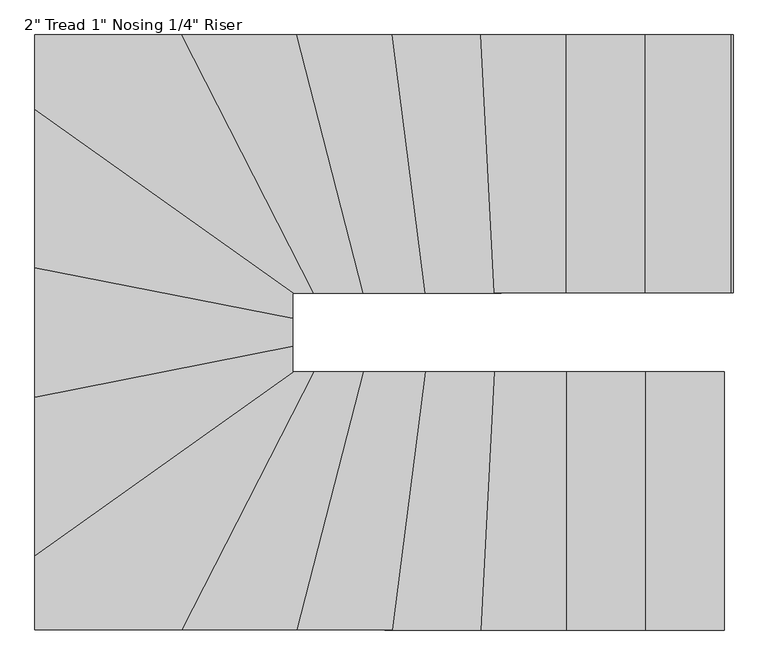
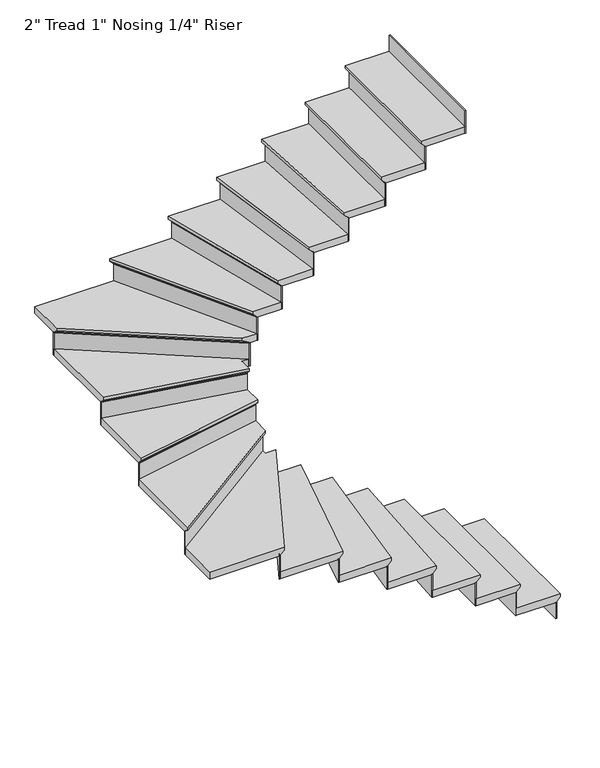
"""IFC4 building model written with IfcOpenShell, lengths in millimetres: stair flight geometry."""

from ifc_helpers import new_model, si_unit, origin, place, context, project, spatial, faceted_brep, source, transform, mapped, element, save


def stair_flight_e7c1aa98(model_context):
    return source(origin(), model_context, "Body", "Brep", [
        faceted_brep([(-14092.4170266, 7781.0465295, 150.2833333), (-14092.4170266, 7781.0465295, 169.3333333), (-14092.4170266, 6866.6465295, 169.3333333), (-14092.4170266, 6866.6465295, 150.2833333), (-14117.8170266, 7781.0465295, 124.8833333), (-14117.8170266, 6866.6465295, 124.8833333), (-14397.2170266, 7781.0465295, 169.3333333), (-14397.2170266, 6866.6465295, 169.3333333), (-14117.8170266, 6866.6465295, 118.5333333), (-14397.2170266, 6866.6465295, 118.5333333), (-14397.2170266, 7781.0465295, 118.5333333), (-14117.8170266, 7781.0465295, 118.5333333)], [[[0, 1, 2, 3]], [[4, 0, 3, 5]], [[2, 1, 6, 7]], [[8, 9, 10, 11]], [[2, 7, 9, 8, 5, 3]], [[8, 11, 4, 5]], [[6, 1, 0, 4, 11, 10]], [[7, 6, 10, 9]]]),
        faceted_brep([(-14117.8170266, 7781.0465295, 118.5333333), (-14117.8170266, 7781.0465295, 0.0), (-14124.1670266, 7781.0465295, 0.0), (-14124.1670266, 7781.0465295, 118.5333333), (-14117.8170266, 6866.6465295, 118.5333333), (-14124.1670266, 6866.6465295, 118.5333333), (-14124.1670266, 6866.6465295, 0.0), (-14117.8170266, 6866.6465295, 0.0)], [[[0, 1, 2, 3]], [[4, 5, 6, 7]], [[1, 0, 4, 7]], [[2, 1, 7, 6]], [[3, 2, 6, 5]], [[0, 3, 5, 4]]]),
        faceted_brep([(-14397.2170266, 7781.0465295, 287.8666667), (-14397.2170266, 7781.0465295, 118.5333333), (-14403.5670266, 7781.0465295, 118.5333333), (-14403.5670266, 7781.0465295, 287.8666667), (-14397.2170266, 6866.6465295, 287.8666667), (-14403.5670266, 6866.6465295, 287.8666667), (-14403.5670266, 6866.6465295, 118.5333333), (-14397.2170266, 6866.6465295, 118.5333333)], [[[0, 1, 2, 3]], [[4, 5, 6, 7]], [[1, 0, 4, 7]], [[2, 1, 7, 6]], [[3, 2, 6, 5]], [[0, 3, 5, 4]]]),
        faceted_brep([(-14371.8170266, 6866.6465295, 338.6666667), (-14371.8170266, 7781.0465295, 338.6666667), (-14676.6170266, 7781.0465295, 338.6666667), (-14676.6170266, 6866.6465295, 338.6666667), (-14397.2170266, 6866.6465295, 287.8666667), (-14676.6170266, 6866.6465295, 287.8666667), (-14676.6170266, 7781.0465295, 287.8666667), (-14397.2170266, 7781.0465295, 287.8666667), (-14397.2170266, 6866.6465295, 294.2166667), (-14371.8170266, 6866.6465295, 319.6166667), (-14397.2170266, 7781.0465295, 294.2166667), (-14371.8170266, 7781.0465295, 319.6166667)], [[[0, 1, 2, 3]], [[4, 5, 6, 7]], [[0, 3, 5, 4, 8, 9]], [[4, 7, 10, 8]], [[2, 1, 11, 10, 7, 6]], [[3, 2, 6, 5]], [[11, 1, 0, 9]], [[10, 11, 9, 8]]]),
        faceted_brep([(-14676.6170266, 7781.0465295, 457.2), (-14676.6170266, 7781.0465295, 287.8666667), (-14682.9670266, 7781.0465295, 287.8666667), (-14682.9670266, 7781.0465295, 457.2), (-14676.6170266, 6866.6465295, 457.2), (-14682.9670266, 6866.6465295, 457.2), (-14682.9670266, 6866.6465295, 287.8666667), (-14676.6170266, 6866.6465295, 287.8666667)], [[[0, 1, 2, 3]], [[4, 5, 6, 7]], [[1, 0, 4, 7]], [[2, 1, 7, 6]], [[3, 2, 6, 5]], [[0, 3, 5, 4]]]),
        faceted_brep([(-14651.2170266, 6866.6465295, 508.0), (-14651.2170266, 7781.0465295, 508.0), (-14932.284188, 7781.0465295, 508.0), (-14979.8184584, 6866.6465295, 508.0), (-14676.6170266, 6866.6465295, 457.2), (-14979.8184584, 6866.6465295, 457.2), (-14932.284188, 7781.0465295, 457.2), (-14676.6170266, 7781.0465295, 457.2), (-14676.6170266, 6866.6465295, 463.55), (-14651.2170266, 6866.6465295, 488.95), (-14676.6170266, 7781.0465295, 463.55), (-14651.2170266, 7781.0465295, 488.95)], [[[0, 1, 2, 3]], [[4, 5, 6, 7]], [[0, 3, 5, 4, 8, 9]], [[4, 7, 10, 8]], [[2, 1, 11, 10, 7, 6]], [[3, 2, 6, 5]], [[11, 1, 0, 9]], [[10, 11, 9, 8]]]),
        faceted_brep([(-14932.284188, 7781.0465295, 626.5333333), (-14932.284188, 7781.0465295, 457.2), (-14938.6427622, 7781.0465295, 457.2), (-14938.6427622, 7781.0465295, 626.5333333), (-14979.8184584, 6866.6465295, 626.5333333), (-14986.1770326, 6866.6465295, 626.5333333), (-14986.1770326, 6866.6465295, 457.2), (-14979.8184584, 6866.6465295, 457.2)], [[[0, 1, 2, 3]], [[4, 5, 6, 7]], [[1, 0, 4, 7]], [[2, 1, 7, 6]], [[3, 2, 6, 5]], [[0, 3, 5, 4]]]),
        faceted_brep([(-14954.3841618, 6866.6465295, 677.3333333), (-14906.8498914, 7781.0465295, 677.3333333), (-15176.4508879, 7781.0465295, 677.3333333), (-15294.8069395, 6866.6465295, 677.3333333), (-14979.8184584, 6866.6465295, 626.5333333), (-15294.8069395, 6866.6465295, 626.5333333), (-15176.4508879, 7781.0465295, 626.5333333), (-14932.284188, 7781.0465295, 626.5333333), (-14979.8184584, 6866.6465295, 632.8833333), (-14954.3841618, 6866.6465295, 658.2833333), (-14932.284188, 7781.0465295, 632.8833333), (-14906.8498914, 7781.0465295, 658.2833333)], [[[0, 1, 2, 3]], [[4, 5, 6, 7]], [[0, 3, 5, 4, 8, 9]], [[4, 7, 10, 8]], [[2, 1, 11, 10, 7, 6]], [[3, 2, 6, 5]], [[11, 1, 0, 9]], [[10, 11, 9, 8]]]),
        faceted_brep([(-15176.4508879, 7781.0465295, 795.8666667), (-15176.4508879, 7781.0465295, 626.5333333), (-15182.8538596, 7781.0465295, 626.5333333), (-15182.8538596, 7781.0465295, 795.8666667), (-15294.8069395, 6866.6465295, 795.8666667), (-15301.2099113, 6866.6465295, 795.8666667), (-15301.2099113, 6866.6465295, 626.5333333), (-15294.8069395, 6866.6465295, 626.5333333)], [[[0, 1, 2, 3]], [[4, 5, 6, 7]], [[1, 0, 4, 7]], [[2, 1, 7, 6]], [[3, 2, 6, 5]], [[0, 3, 5, 4]]]),
        faceted_brep([(-15269.1950524, 6866.6465295, 846.6666667), (-15150.8390007, 7781.0465295, 846.6666667), (-15398.0781103, 7781.0465295, 846.6666667), (-15633.2085577, 6866.6465295, 846.6666667), (-15294.8069395, 6866.6465295, 795.8666667), (-15633.2085577, 6866.6465295, 795.8666667), (-15398.0781103, 7781.0465295, 795.8666667), (-15176.4508879, 7781.0465295, 795.8666667), (-15294.8069395, 6866.6465295, 802.2166667), (-15269.1950524, 6866.6465295, 827.6166667), (-15176.4508879, 7781.0465295, 802.2166667), (-15150.8390007, 7781.0465295, 827.6166667)], [[[0, 1, 2, 3]], [[4, 5, 6, 7]], [[0, 3, 5, 4, 8, 9]], [[4, 7, 10, 8]], [[2, 1, 11, 10, 7, 6]], [[3, 2, 6, 5]], [[11, 1, 0, 9]], [[10, 11, 9, 8]]]),
        faceted_brep([(-15398.0781103, 7781.0465295, 965.2), (-15398.0781103, 7781.0465295, 795.8666667), (-15404.6346872, 7781.0465295, 795.8666667), (-15404.6346872, 7781.0465295, 965.2), (-15633.2085577, 6866.6465295, 965.2), (-15639.7651346, 6866.6465295, 965.2), (-15639.7651346, 6866.6465295, 795.8666667), (-15633.2085577, 6866.6465295, 795.8666667)], [[[0, 1, 2, 3]], [[4, 5, 6, 7]], [[1, 0, 4, 7]], [[2, 1, 7, 6]], [[3, 2, 6, 5]], [[0, 3, 5, 4]]]),
        faceted_brep([(-15606.9822503, 6866.6465295, 1016.0), (-15371.8518029, 7781.0465295, 1016.0), (-15574.4247464, 7781.0465295, 1016.0), (-16043.2493677, 6866.6465295, 1016.0), (-15633.2085577, 6866.6465295, 965.2), (-16043.2493677, 6866.6465295, 965.2), (-15574.4247464, 7781.0465295, 965.2), (-15398.0781103, 7781.0465295, 965.2), (-15633.2085577, 6866.6465295, 971.55), (-15606.9822503, 6866.6465295, 996.95), (-15398.0781103, 7781.0465295, 971.55), (-15371.8518029, 7781.0465295, 996.95)], [[[0, 1, 2, 3]], [[4, 5, 6, 7]], [[0, 3, 5, 4, 8, 9]], [[4, 7, 10, 8]], [[2, 1, 11, 10, 7, 6]], [[3, 2, 6, 5]], [[11, 1, 0, 9]], [[10, 11, 9, 8]]]),
        faceted_brep([(-15574.4247464, 7781.0465295, 1134.5333333), (-15574.4247464, 7781.0465295, 965.2), (-15581.5607295, 7781.0465295, 965.2), (-15581.5607295, 7781.0465295, 1134.5333333), (-16043.2493677, 6866.6465295, 1134.5333333), (-16050.3853509, 6866.6465295, 1134.5333333), (-16050.3853509, 6866.6465295, 965.2), (-16043.2493677, 6866.6465295, 965.2)], [[[0, 1, 2, 3]], [[4, 5, 6, 7]], [[1, 0, 4, 7]], [[2, 1, 7, 6]], [[3, 2, 6, 5]], [[0, 3, 5, 4]]]),
        faceted_brep([(-16534.5487184, 7160.3276632, 1185.3333333), (-16534.5487184, 6866.6465295, 1185.3333333), (-16014.7054352, 6866.6465295, 1185.3333333), (-15545.8808139, 7781.0465295, 1185.3333333), (-15620.1487184, 7781.0465295, 1185.3333333), (-15620.1487184, 7810.6016123, 1185.3333333), (-16534.5487184, 6866.6465295, 1134.5333333), (-16534.5487184, 7160.3276632, 1134.5333333), (-15620.1487184, 7810.6016123, 1134.5333333), (-15620.1487184, 7781.0465295, 1134.5333333), (-15574.4247464, 7781.0465295, 1134.5333333), (-16043.2493677, 6866.6465295, 1134.5333333), (-16043.2493677, 6866.6465295, 1140.8833333), (-16014.7054352, 6866.6465295, 1166.2833333), (-15574.4247464, 7781.0465295, 1140.8833333), (-15545.8808139, 7781.0465295, 1166.2833333)], [[[0, 1, 2, 3, 4, 5]], [[6, 7, 8, 9, 10, 11]], [[1, 0, 7, 6]], [[2, 1, 6, 11, 12, 13]], [[11, 10, 14, 12]], [[4, 3, 15, 14, 10, 9]], [[5, 4, 9, 8]], [[0, 5, 8, 7]], [[15, 3, 2, 13]], [[14, 15, 13, 12]]]),
        faceted_brep([(-15620.1487184, 7810.6016123, 1303.8666667), (-15620.1487184, 7810.6016123, 1134.5333333), (-15620.1487184, 7818.3935871, 1134.5333333), (-15620.1487184, 7818.3935871, 1303.8666667), (-16534.5487184, 7160.3276632, 1303.8666667), (-16534.5487184, 7168.1196379, 1303.8666667), (-16534.5487184, 7168.1196379, 1134.5333333), (-16534.5487184, 7160.3276632, 1134.5333333)], [[[0, 1, 2, 3]], [[4, 5, 6, 7]], [[1, 0, 4, 7]], [[2, 1, 7, 6]], [[3, 2, 6, 5]], [[0, 3, 5, 4]]]),
        faceted_brep([(-16534.5487184, 7129.159764, 1354.6666667), (-15620.1487184, 7779.4337131, 1354.6666667), (-15620.1487184, 7897.0556994, 1354.6666667), (-16534.5487184, 7716.814843, 1354.6666667), (-16534.5487184, 7160.3276632, 1303.8666667), (-16534.5487184, 7716.814843, 1303.8666667), (-15620.1487184, 7897.0556994, 1303.8666667), (-15620.1487184, 7810.6016123, 1303.8666667), (-16534.5487184, 7160.3276632, 1310.2166667), (-16534.5487184, 7129.159764, 1335.6166667), (-15620.1487184, 7810.6016123, 1310.2166667), (-15620.1487184, 7779.4337131, 1335.6166667)], [[[0, 1, 2, 3]], [[4, 5, 6, 7]], [[0, 3, 5, 4, 8, 9]], [[4, 7, 10, 8]], [[2, 1, 11, 10, 7, 6]], [[3, 2, 6, 5]], [[11, 1, 0, 9]], [[10, 11, 9, 8]]]),
        faceted_brep([(-15620.1487184, 7897.0556994, 1473.2), (-15620.1487184, 7897.0556994, 1303.8666667), (-15620.1487184, 7903.5278848, 1303.8666667), (-15620.1487184, 7903.5278848, 1473.2), (-16534.5487184, 7716.814843, 1473.2), (-16534.5487184, 7723.2870285, 1473.2), (-16534.5487184, 7723.2870285, 1303.8666667), (-16534.5487184, 7716.814843, 1303.8666667)], [[[0, 1, 2, 3]], [[4, 5, 6, 7]], [[1, 0, 4, 7]], [[2, 1, 7, 6]], [[3, 2, 6, 5]], [[0, 3, 5, 4]]]),
        faceted_brep([(-16534.5487184, 7690.9261013, 1524.0), (-15620.1487184, 7871.1669576, 1524.0), (-15620.1487184, 7996.214843, 1524.0), (-16534.5487184, 8176.4556994, 1524.0), (-16534.5487184, 7716.814843, 1473.2), (-16534.5487184, 8176.4556994, 1473.2), (-15620.1487184, 7996.214843, 1473.2), (-15620.1487184, 7897.0556994, 1473.2), (-16534.5487184, 7716.814843, 1479.55), (-16534.5487184, 7690.9261013, 1504.95), (-15620.1487184, 7897.0556994, 1479.55), (-15620.1487184, 7871.1669576, 1504.95)], [[[0, 1, 2, 3]], [[4, 5, 6, 7]], [[0, 3, 5, 4, 8, 9]], [[4, 7, 10, 8]], [[2, 1, 11, 10, 7, 6]], [[3, 2, 6, 5]], [[11, 1, 0, 9]], [[10, 11, 9, 8]]]),
        faceted_brep([(-15620.1487184, 7996.214843, 1642.5333333), (-15620.1487184, 7996.214843, 1473.2), (-15620.1487184, 8002.6870285, 1473.2), (-15620.1487184, 8002.6870285, 1642.5333333), (-16534.5487184, 8176.4556994, 1642.5333333), (-16534.5487184, 8182.9278848, 1642.5333333), (-16534.5487184, 8182.9278848, 1473.2), (-16534.5487184, 8176.4556994, 1473.2)], [[[0, 1, 2, 3]], [[4, 5, 6, 7]], [[1, 0, 4, 7]], [[2, 1, 7, 6]], [[3, 2, 6, 5]], [[0, 3, 5, 4]]]),
        faceted_brep([(-16534.5487184, 8150.5669576, 1693.3333333), (-15620.1487184, 7970.3261013, 1693.3333333), (-15620.1487184, 8060.4465295, 1693.3333333), (-15574.0532439, 8060.4465295, 1693.3333333), (-16534.5487184, 8743.5011941, 1693.3333333), (-16534.5487184, 8176.4556994, 1642.5333333), (-16534.5487184, 8743.5011941, 1642.5333333), (-15574.0532439, 8060.4465295, 1642.5333333), (-15620.1487184, 8060.4465295, 1642.5333333), (-15620.1487184, 7996.214843, 1642.5333333), (-16534.5487184, 8176.4556994, 1648.8833333), (-16534.5487184, 8150.5669576, 1674.2833333), (-15620.1487184, 7996.214843, 1648.8833333), (-15620.1487184, 7970.3261013, 1674.2833333)], [[[0, 1, 2, 3, 4]], [[5, 6, 7, 8, 9]], [[0, 4, 6, 5, 10, 11]], [[5, 9, 12, 10]], [[2, 1, 13, 12, 9, 8]], [[3, 2, 8, 7]], [[4, 3, 7, 6]], [[13, 1, 0, 11]], [[12, 13, 11, 10]]]),
        faceted_brep([(-15574.0532439, 8060.4465295, 1811.8666667), (-15574.0532439, 8060.4465295, 1642.5333333), (-15563.0963514, 8060.4465295, 1642.5333333), (-15563.0963514, 8060.4465295, 1811.8666667), (-16534.5487184, 8743.5011941, 1811.8666667), (-16534.5487184, 8751.2931689, 1811.8666667), (-16534.5487184, 8751.2931689, 1642.5333333), (-16534.5487184, 8743.5011941, 1642.5333333)], [[[0, 1, 2, 3]], [[4, 5, 6, 7]], [[1, 0, 4, 7]], [[2, 1, 7, 6]], [[3, 2, 6, 5]], [[0, 3, 5, 4]]]),
        faceted_brep([(-15986.1615027, 8974.8465295, 1862.6666667), (-16534.5487184, 8974.8465295, 1862.6666667), (-16534.5487184, 8712.3332949, 1862.6666667), (-15617.8808139, 8060.4465295, 1862.6666667), (-15517.3368813, 8060.4465295, 1862.6666667), (-16534.5487184, 8974.8465295, 1811.8666667), (-15986.1615027, 8974.8465295, 1811.8666667), (-15517.3368813, 8060.4465295, 1811.8666667), (-15574.0532439, 8060.4465295, 1811.8666667), (-16534.5487184, 8743.5011941, 1811.8666667), (-16534.5487184, 8743.5011941, 1818.2166667), (-16534.5487184, 8712.3332949, 1843.6166667), (-15574.0532439, 8060.4465295, 1818.2166667), (-15617.8808139, 8060.4465295, 1843.6166667)], [[[0, 1, 2, 3, 4]], [[5, 6, 7, 8, 9]], [[1, 0, 6, 5]], [[2, 1, 5, 9, 10, 11]], [[9, 8, 12, 10]], [[4, 3, 13, 12, 8, 7]], [[0, 4, 7, 6]], [[13, 3, 2, 11]], [[12, 13, 11, 10]]]),
        faceted_brep([(-15517.3368813, 8060.4465295, 1981.2), (-15517.3368813, 8060.4465295, 1811.8666667), (-15510.2008982, 8060.4465295, 1811.8666667), (-15510.2008982, 8060.4465295, 1981.2), (-15986.1615027, 8974.8465295, 1981.2), (-15979.0255195, 8974.8465295, 1981.2), (-15979.0255195, 8974.8465295, 1811.8666667), (-15986.1615027, 8974.8465295, 1811.8666667)], [[[0, 1, 2, 3]], [[4, 5, 6, 7]], [[1, 0, 4, 7]], [[2, 1, 7, 6]], [[3, 2, 6, 5]], [[0, 3, 5, 4]]]),
        faceted_brep([(-16014.7054352, 8974.8465295, 2032.0), (-15545.8808139, 8060.4465295, 2032.0), (-15345.6254954, 8060.4465295, 2032.0), (-15580.7559428, 8974.8465295, 2032.0), (-15986.1615027, 8974.8465295, 1981.2), (-15580.7559428, 8974.8465295, 1981.2), (-15345.6254954, 8060.4465295, 1981.2), (-15517.3368813, 8060.4465295, 1981.2), (-15986.1615027, 8974.8465295, 1987.55), (-16014.7054352, 8974.8465295, 2012.95), (-15517.3368813, 8060.4465295, 1987.55), (-15545.8808139, 8060.4465295, 2012.95)], [[[0, 1, 2, 3]], [[4, 5, 6, 7]], [[0, 3, 5, 4, 8, 9]], [[4, 7, 10, 8]], [[2, 1, 11, 10, 7, 6]], [[3, 2, 6, 5]], [[11, 1, 0, 9]], [[10, 11, 9, 8]]]),
        faceted_brep([(-15345.6254954, 8060.4465295, 2150.5333333), (-15345.6254954, 8060.4465295, 1981.2), (-15339.0689185, 8060.4465295, 1981.2), (-15339.0689185, 8060.4465295, 2150.5333333), (-15580.7559428, 8974.8465295, 2150.5333333), (-15574.1993659, 8974.8465295, 2150.5333333), (-15574.1993659, 8974.8465295, 1981.2), (-15580.7559428, 8974.8465295, 1981.2)], [[[0, 1, 2, 3]], [[4, 5, 6, 7]], [[1, 0, 4, 7]], [[2, 1, 7, 6]], [[3, 2, 6, 5]], [[0, 3, 5, 4]]]),
        faceted_brep([(-15606.9822503, 8974.8465295, 2201.3333333), (-15371.8518029, 8060.4465295, 2201.3333333), (-15125.2271136, 8060.4465295, 2201.3333333), (-15243.5831653, 8974.8465295, 2201.3333333), (-15580.7559428, 8974.8465295, 2150.5333333), (-15243.5831653, 8974.8465295, 2150.5333333), (-15125.2271136, 8060.4465295, 2150.5333333), (-15345.6254954, 8060.4465295, 2150.5333333), (-15580.7559428, 8974.8465295, 2156.8833333), (-15606.9822503, 8974.8465295, 2182.2833333), (-15345.6254954, 8060.4465295, 2156.8833333), (-15371.8518029, 8060.4465295, 2182.2833333)], [[[0, 1, 2, 3]], [[4, 5, 6, 7]], [[0, 3, 5, 4, 8, 9]], [[4, 7, 10, 8]], [[2, 1, 11, 10, 7, 6]], [[3, 2, 6, 5]], [[11, 1, 0, 9]], [[10, 11, 9, 8]]]),
        faceted_brep([(-15125.2271136, 8060.4465295, 2319.8666667), (-15125.2271136, 8060.4465295, 2150.5333333), (-15118.8241418, 8060.4465295, 2150.5333333), (-15118.8241418, 8060.4465295, 2319.8666667), (-15243.5831653, 8974.8465295, 2319.8666667), (-15237.1801935, 8974.8465295, 2319.8666667), (-15237.1801935, 8974.8465295, 2150.5333333), (-15243.5831653, 8974.8465295, 2150.5333333)], [[[0, 1, 2, 3]], [[4, 5, 6, 7]], [[1, 0, 4, 7]], [[2, 1, 7, 6]], [[3, 2, 6, 5]], [[0, 3, 5, 4]]]),
        faceted_brep([(-15269.1950524, 8974.8465295, 2370.6666667), (-15150.8390007, 8060.4465295, 2370.6666667), (-14881.4155947, 8060.4465295, 2370.6666667), (-14928.9498651, 8974.8465295, 2370.6666667), (-15243.5831653, 8974.8465295, 2319.8666667), (-14928.9498651, 8974.8465295, 2319.8666667), (-14881.4155947, 8060.4465295, 2319.8666667), (-15125.2271136, 8060.4465295, 2319.8666667), (-15243.5831653, 8974.8465295, 2326.2166667), (-15269.1950524, 8974.8465295, 2351.6166667), (-15125.2271136, 8060.4465295, 2326.2166667), (-15150.8390007, 8060.4465295, 2351.6166667)], [[[0, 1, 2, 3]], [[4, 5, 6, 7]], [[0, 3, 5, 4, 8, 9]], [[4, 7, 10, 8]], [[2, 1, 11, 10, 7, 6]], [[3, 2, 6, 5]], [[11, 1, 0, 9]], [[10, 11, 9, 8]]]),
        faceted_brep([(-14881.4155947, 8060.4465295, 2489.2), (-14881.4155947, 8060.4465295, 2319.8666667), (-14875.0570205, 8060.4465295, 2319.8666667), (-14875.0570205, 8060.4465295, 2489.2), (-14928.9498651, 8974.8465295, 2489.2), (-14922.5912909, 8974.8465295, 2489.2), (-14922.5912909, 8974.8465295, 2319.8666667), (-14928.9498651, 8974.8465295, 2319.8666667)], [[[0, 1, 2, 3]], [[4, 5, 6, 7]], [[1, 0, 4, 7]], [[2, 1, 7, 6]], [[3, 2, 6, 5]], [[0, 3, 5, 4]]]),
        faceted_brep([(-14954.3841618, 8974.8465295, 2540.0), (-14906.8498914, 8060.4465295, 2540.0), (-14625.8170266, 8060.4465295, 2540.0), (-14625.8170266, 8974.8465295, 2540.0), (-14928.9498651, 8974.8465295, 2489.2), (-14625.8170266, 8974.8465295, 2489.2), (-14625.8170266, 8060.4465295, 2489.2), (-14881.4155947, 8060.4465295, 2489.2), (-14928.9498651, 8974.8465295, 2495.55), (-14954.3841618, 8974.8465295, 2520.95), (-14881.4155947, 8060.4465295, 2495.55), (-14906.8498914, 8060.4465295, 2520.95)], [[[0, 1, 2, 3]], [[4, 5, 6, 7]], [[0, 3, 5, 4, 8, 9]], [[4, 7, 10, 8]], [[2, 1, 11, 10, 7, 6]], [[3, 2, 6, 5]], [[11, 1, 0, 9]], [[10, 11, 9, 8]]]),
        faceted_brep([(-14625.8170266, 8060.4465295, 2658.5333333), (-14625.8170266, 8060.4465295, 2489.2), (-14619.4670266, 8060.4465295, 2489.2), (-14619.4670266, 8060.4465295, 2658.5333333), (-14625.8170266, 8974.8465295, 2658.5333333), (-14619.4670266, 8974.8465295, 2658.5333333), (-14619.4670266, 8974.8465295, 2489.2), (-14625.8170266, 8974.8465295, 2489.2)], [[[0, 1, 2, 3]], [[4, 5, 6, 7]], [[1, 0, 4, 7]], [[2, 1, 7, 6]], [[3, 2, 6, 5]], [[0, 3, 5, 4]]]),
        faceted_brep([(-14651.2170266, 8974.8465295, 2709.3333333), (-14651.2170266, 8060.4465295, 2709.3333333), (-14346.4170266, 8060.4465295, 2709.3333333), (-14346.4170266, 8974.8465295, 2709.3333333), (-14625.8170266, 8974.8465295, 2658.5333333), (-14346.4170266, 8974.8465295, 2658.5333333), (-14346.4170266, 8060.4465295, 2658.5333333), (-14625.8170266, 8060.4465295, 2658.5333333), (-14625.8170266, 8974.8465295, 2664.8833333), (-14651.2170266, 8974.8465295, 2690.2833333), (-14625.8170266, 8060.4465295, 2664.8833333), (-14651.2170266, 8060.4465295, 2690.2833333)], [[[0, 1, 2, 3]], [[4, 5, 6, 7]], [[0, 3, 5, 4, 8, 9]], [[4, 7, 10, 8]], [[2, 1, 11, 10, 7, 6]], [[3, 2, 6, 5]], [[11, 1, 0, 9]], [[10, 11, 9, 8]]]),
        faceted_brep([(-14346.4170266, 8060.4465295, 2827.8666667), (-14346.4170266, 8060.4465295, 2658.5333333), (-14340.0670266, 8060.4465295, 2658.5333333), (-14340.0670266, 8060.4465295, 2827.8666667), (-14346.4170266, 8974.8465295, 2827.8666667), (-14340.0670266, 8974.8465295, 2827.8666667), (-14340.0670266, 8974.8465295, 2658.5333333), (-14346.4170266, 8974.8465295, 2658.5333333)], [[[0, 1, 2, 3]], [[4, 5, 6, 7]], [[1, 0, 4, 7]], [[2, 1, 7, 6]], [[3, 2, 6, 5]], [[0, 3, 5, 4]]]),
        faceted_brep([(-14067.0170266, 8060.4465295, 2997.2), (-14067.0170266, 8060.4465295, 2827.8666667), (-14060.6670266, 8060.4465295, 2827.8666667), (-14060.6670266, 8060.4465295, 2997.2), (-14067.0170266, 8974.8465295, 2997.2), (-14060.6670266, 8974.8465295, 2997.2), (-14060.6670266, 8974.8465295, 2827.8666667), (-14067.0170266, 8974.8465295, 2827.8666667)], [[[0, 1, 2, 3]], [[4, 5, 6, 7]], [[1, 0, 4, 7]], [[2, 1, 7, 6]], [[3, 2, 6, 5]], [[0, 3, 5, 4]]]),
        faceted_brep([(-14371.8170266, 8974.8465295, 2878.6666667), (-14371.8170266, 8060.4465295, 2878.6666667), (-14067.0170266, 8060.4465295, 2878.6666667), (-14067.0170266, 8974.8465295, 2878.6666667), (-14346.4170266, 8974.8465295, 2827.8666667), (-14067.0170266, 8974.8465295, 2827.8666667), (-14067.0170266, 8060.4465295, 2827.8666667), (-14346.4170266, 8060.4465295, 2827.8666667), (-14346.4170266, 8974.8465295, 2834.2166667), (-14371.8170266, 8974.8465295, 2859.6166667), (-14346.4170266, 8060.4465295, 2834.2166667), (-14371.8170266, 8060.4465295, 2859.6166667)], [[[0, 1, 2, 3]], [[4, 5, 6, 7]], [[0, 3, 5, 4, 8, 9]], [[4, 7, 10, 8]], [[2, 1, 11, 10, 7, 6]], [[3, 2, 6, 5]], [[11, 1, 0, 9]], [[10, 11, 9, 8]]]),
    ])


if __name__ == "__main__":
    model = new_model("IFC4")
    model_context = context("Model", 3, world=origin())
    ifc_project = project(units=[si_unit("LENGTHUNIT", "METRE", prefix="MILLI")], contexts=[model_context])
    site = spatial("IfcSite", under=ifc_project)
    building = spatial("IfcBuilding", under=site)
    placement = place(None, origin())
    stair_flight_shape = stair_flight_e7c1aa98(model_context)
    element("IfcStairFlight", 1, ObjectType="2\" Tread 1\" Nosing 1/4\" Riser", at=placement, inside=building, context=model_context, shape_type="MappedRepresentation", body=[
        mapped(stair_flight_shape, transform((0.0, 0.0, 0.0), x_axis=(1.0, 0.0, 0.0), y_axis=(0.0, 1.0, 0.0), z_axis=(0.0, 0.0, 1.0))),
    ])
    save(model, "model.ifc")
